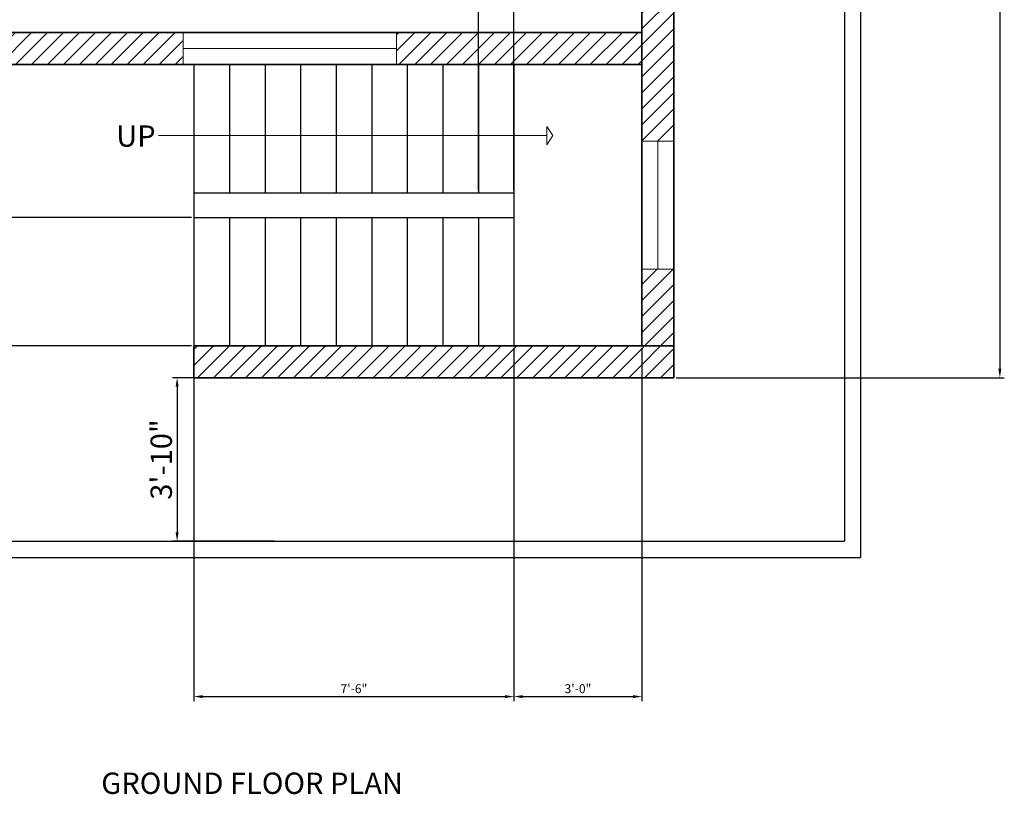
# Model space of a CAD drawing. Units: inches. Extents: x 3618 to 4156, y 1271 to 2023.
# Tile 2 of 5: x 3879 to 4156, y 1271 to 1488. Entities that reach past the tile are written whole.
import ezdxf

# ---------------------------------------------------------------- set-up
doc = ezdxf.new("R2010")
doc.units = ezdxf.units.IN
for name, color, linetype, lineweight in [('A-ANNO-DIMS', 2, 'Continuous', 18), ('A-ANNO-SYMB', 7, 'Continuous', 18), ('A-ANNO-TEXT', 7, 'Continuous', 18), ('A-ANNO-TITL', 7, 'Continuous', 25), ('A-FLOR-STRS', 7, 'Continuous', 25), ('A-GLAZ', 4, 'Continuous', 18), ('A-WALL', 7, 'Continuous', 35), ('A-WALL-PATT', 252, 'Continuous', 13), ('C-PROP', 7, 'Continuous', 25)]:
    doc.layers.add(name, color=color, linetype=linetype, lineweight=lineweight)
doc.styles.get("Standard").update_dxf_attribs({"font": 'arial.ttf'})
doc.dimstyles.new('ISO-25', dxfattribs={"dimtxt": 2.5, "dimasz": 2.5, "dimexe": 1.25, "dimexo": 0.625, "dimtad": 1, "dimdec": 0, "dimlunit": 3, "dimtxsty": 'Standard', "dimcen": 2.5, "dimadec": 0, "dimazin": 0, "dimtfac": 1, "dimtdec": 0, "dimtmove": 0, "dimatfit": 3, "dimfxl": 1, "dimarcsym": 0})

# ---------------------------------------------------------------- blocks, each defined once
blk = doc.blocks.new('*D2')
at = {"layer": 'A-ANNO-DIMS', "color": 0, "lineweight": -2, "transparency": 16777216}
for p, q in [((3942.74, 1387.81), (3922.22, 1387.81)), ((3923.47, 1385.31), (3923.47, 1344.31)), ((3950.79, 1341.81), (3922.22, 1341.81))]:
    blk.add_line(p, q, dxfattribs=at)
at = {"layer": 'A-ANNO-DIMS', "color": 0, "transparency": 16777216}
for points in [[(3923.05, 1385.31), (3923.88, 1385.31), (3923.47, 1387.81)], [(3923.05, 1344.31), (3923.88, 1344.31), (3923.47, 1341.81)]]:
    blk.add_solid(points, dxfattribs=at)
at = {"layer": 'Defpoints', "color": 0, "transparency": 16777216}
for p in [(3943.36, 1387.81), (3923.47, 1341.81), (3951.41, 1341.81)]:
    blk.add_point(p, dxfattribs=at)
at = {"layer": 'A-ANNO-DIMS', "color": 0, "transparency": 16777216, "insert": (3919.78, 1364.81), "char_height": 6, "attachment_point": 5, "rotation": 90}
blk.add_mtext('3\'-10"', dxfattribs=at)
blk = doc.blocks.new('WINDOW-36X9')
for p, q in [((0, 36), (0, 0)), ((9, 36), (0, 36)), ((4.5, 36), (4.5, 0)), ((9, 0), (9, 36)), ((0, 0), (9, 0))]:
    blk.add_line(p, q)
blk = doc.blocks.new('WINDOW-60X9')
for p, q in [((0, 60), (0, 0)), ((9, 60), (0, 60)), ((4.5, 60), (4.5, 0)), ((9, 0), (9, 60)), ((0, 0), (9, 0))]:
    blk.add_line(p, q)
blk = doc.blocks.new('*D50')
at = {"layer": 'A-ANNO-DIMS', "color": 0, "lineweight": -2, "transparency": 16777216}
for p, q in [((3928.19, 1396.19), (3928.19, 1296.91)), ((4018.19, 1396.19), (4018.19, 1296.91)), ((3930.69, 1298.16), (4015.69, 1298.16))]:
    blk.add_line(p, q, dxfattribs=at)
at = {"layer": 'A-ANNO-DIMS', "color": 0, "transparency": 16777216}
for points in [[(3930.69, 1298.58), (3930.69, 1297.74), (3928.19, 1298.16)], [(4015.69, 1298.58), (4015.69, 1297.74), (4018.19, 1298.16)]]:
    blk.add_solid(points, dxfattribs=at)
at = {"layer": 'Defpoints', "color": 0, "transparency": 16777216}
for p in [(3928.19, 1396.81), (4018.19, 1396.81), (4018.19, 1298.16)]:
    blk.add_point(p, dxfattribs=at)
at = {"layer": 'A-ANNO-DIMS', "color": 0, "transparency": 16777216, "insert": (3973.19, 1300.06), "char_height": 2.5, "attachment_point": 5}
blk.add_mtext('7\'-6"', dxfattribs=at)
blk = doc.blocks.new('*D51')
at = {"layer": 'A-ANNO-DIMS', "color": 0, "lineweight": -2, "transparency": 16777216}
for p, q in [((4018.19, 1396.19), (4018.19, 1296.91)), ((4054.19, 1396.19), (4054.19, 1296.91)), ((4020.69, 1298.16), (4051.69, 1298.16))]:
    blk.add_line(p, q, dxfattribs=at)
at = {"layer": 'A-ANNO-DIMS', "color": 0, "transparency": 16777216}
for points in [[(4020.69, 1298.58), (4020.69, 1297.74), (4018.19, 1298.16)], [(4051.69, 1298.58), (4051.69, 1297.74), (4054.19, 1298.16)]]:
    blk.add_solid(points, dxfattribs=at)
at = {"layer": 'Defpoints', "color": 0, "transparency": 16777216}
for p in [(4018.19, 1396.81), (4054.19, 1396.81), (4054.19, 1298.16)]:
    blk.add_point(p, dxfattribs=at)
at = {"layer": 'A-ANNO-DIMS', "color": 0, "transparency": 16777216, "insert": (4036.19, 1300.06), "char_height": 2.5, "attachment_point": 5}
blk.add_mtext('3\'-0"', dxfattribs=at)
blk = doc.blocks.new('*D52')
at = {"layer": 'A-ANNO-DIMS', "color": 0, "lineweight": -2, "transparency": 16777216}
for p, q in [((3927.56, 1432.81), (3622.79, 1432.81)), ((3624.04, 1399.31), (3624.04, 1430.31)), ((3927.56, 1396.81), (3622.79, 1396.81))]:
    blk.add_line(p, q, dxfattribs=at)
at = {"layer": 'A-ANNO-DIMS', "color": 0, "transparency": 16777216}
for points in [[(3623.62, 1430.31), (3624.45, 1430.31), (3624.04, 1432.81)], [(3623.62, 1399.31), (3624.45, 1399.31), (3624.04, 1396.81)]]:
    blk.add_solid(points, dxfattribs=at)
at = {"layer": 'Defpoints', "color": 0, "transparency": 16777216}
for p in [(3624.04, 1432.81), (3928.19, 1432.81), (3928.19, 1396.81)]:
    blk.add_point(p, dxfattribs=at)
at = {"layer": 'A-ANNO-DIMS', "color": 0, "transparency": 16777216, "insert": (3622.14, 1414.81), "char_height": 2.5, "attachment_point": 5, "rotation": 90}
blk.add_mtext('3\'-0"', dxfattribs=at)
blk = doc.blocks.new('*D53')
at = {"layer": 'A-ANNO-DIMS', "color": 0, "lineweight": -2, "transparency": 16777216}
for p, q in [((4008.19, 1440.44), (4008.19, 1974.21)), ((4018.19, 1440.44), (4018.19, 1974.21)), ((4010.69, 1972.96), (4015.69, 1972.96))]:
    blk.add_line(p, q, dxfattribs=at)
at = {"layer": 'A-ANNO-DIMS', "color": 0, "transparency": 16777216}
for points in [[(4010.69, 1973.38), (4010.69, 1972.54), (4008.19, 1972.96)], [(4015.69, 1973.38), (4015.69, 1972.54), (4018.19, 1972.96)]]:
    blk.add_solid(points, dxfattribs=at)
at = {"layer": 'Defpoints', "color": 0, "transparency": 16777216}
for p in [(4018.19, 1972.96), (4008.19, 1439.81), (4018.19, 1439.81)]:
    blk.add_point(p, dxfattribs=at)
at = {"layer": 'A-ANNO-DIMS', "color": 0, "transparency": 16777216, "insert": (4013.19, 1974.86), "char_height": 2.5, "attachment_point": 5}
blk.add_mtext('0\'-10"', dxfattribs=at)
blk = doc.blocks.new('*D56')
at = {"layer": 'A-ANNO-DIMS', "color": 0, "lineweight": -2, "transparency": 16777216}
for p, q in [((4063.81, 1831.81), (4156.09, 1831.81)), ((4154.84, 1829.31), (4154.84, 1390.31)), ((4063.81, 1387.81), (4156.09, 1387.81))]:
    blk.add_line(p, q, dxfattribs=at)
at = {"layer": 'A-ANNO-DIMS', "color": 0, "transparency": 16777216}
for points in [[(4154.42, 1829.31), (4155.25, 1829.31), (4154.84, 1831.81)], [(4154.42, 1390.31), (4155.25, 1390.31), (4154.84, 1387.81)]]:
    blk.add_solid(points, dxfattribs=at)
at = {"layer": 'Defpoints', "color": 0, "transparency": 16777216}
for p in [(4063.19, 1831.81), (4063.19, 1387.81), (4154.84, 1387.81)]:
    blk.add_point(p, dxfattribs=at)
at = {"layer": 'A-ANNO-DIMS', "color": 0, "transparency": 16777216, "insert": (4152.94, 1609.81), "char_height": 2.5, "attachment_point": 5, "rotation": 90}
blk.add_mtext('37\'-0"', dxfattribs=at)

msp = doc.modelspace()

# ---------------------------------------------------------------- hatches: boundary and pattern name
at = {"layer": 'A-WALL-PATT'}
h = msp.add_hatch(dxfattribs=at)
h.set_pattern_fill('ANSI31', color=256)
h.paths.add_polyline_path([(4115.69, 1933.81), (3704.69, 1933.81), (3704.69, 1885.81), (3713.69, 1885.81), (3713.69, 1924.81), (4115.69, 1924.81)])
h.paths.add_polyline_path([(3886.19, 1924.81), (3881.69, 1924.81), (3881.69, 1786.81), (3875.69, 1786.81), (3875.69, 1782.31), (3892.19, 1782.31), (3892.19, 1786.81), (3886.19, 1786.81)])
h.paths.add_polyline_path([(3763.69, 1784.56), (3763.69, 1786.81), (3713.69, 1786.81), (3713.69, 1782.31), (3763.69, 1782.31)], flags=17)
h.paths.add_polyline_path([(3713.69, 1825.81), (3704.69, 1825.81), (3704.69, 1764.31), (3713.69, 1764.31)])
h.paths.add_polyline_path([(3802.19, 1782.31), (3835.69, 1782.31), (3835.69, 1784.56), (3835.69, 1786.81), (3791.69, 1786.81), (3791.69, 1782.31), (3797.69, 1782.31), (3797.69, 1722.31), (3713.69, 1722.31), (3713.69, 1717.81), (3797.69, 1717.81), (3797.69, 1657.81), (3791.69, 1657.81), (3791.69, 1653.31), (3851.69, 1653.31), (3851.69, 1647.31), (3856.19, 1647.31), (3856.19, 1657.81), (3802.19, 1657.81)])
h.paths.add_polyline_path([(3713.69, 1740.31), (3704.69, 1740.31), (3704.69, 1699.81), (3713.69, 1699.81)])
h.paths.add_polyline_path([(3713.69, 1675.81), (3704.69, 1675.81), (3704.69, 1623.31), (3713.69, 1623.31)])
h.paths.add_polyline_path([(3743.18, 1533.31), (3713.69, 1533.31), (3713.69, 1563.31), (3704.69, 1563.31), (3704.69, 1524.31), (3743.18, 1524.31)])
h.paths.add_polyline_path([(3856.19, 1533.31), (3803.18, 1533.31), (3803.18, 1524.31), (3847.19, 1524.31), (3847.19, 1518.31), (3856.19, 1518.31)])
h.paths.add_polyline_path([(3856.19, 1607.31), (3853.94, 1607.31), (3851.69, 1607.31), (3851.69, 1533.31), (3856.19, 1533.31)])
h.paths.add_polyline_path([(3763.69, 1655.56), (3763.69, 1657.81), (3713.69, 1657.81), (3713.69, 1653.31), (3763.69, 1653.31)], flags=17)
h.paths.add_polyline_path([(4063.19, 1670.56), (4054.19, 1670.56), (4054.19, 1645.31), (3940.98, 1645.31), (3940.98, 1640.81), (4054.19, 1640.81), (4054.19, 1592.81), (4063.19, 1592.81)])
h.paths.add_polyline_path([(4063.19, 1532.81), (4054.19, 1532.81), (4054.19, 1454.31), (4063.19, 1454.31)])
h.paths.add_polyline_path([(4054.19, 1484.81), (3985.19, 1484.81), (3985.19, 1475.81), (4054.19, 1475.81)])
h.paths.add_polyline_path([(3925.19, 1484.81), (3856.19, 1484.81), (3856.19, 1490.81), (3847.19, 1490.81), (3847.19, 1475.81), (3925.19, 1475.81)])
h.paths.add_polyline_path([(4063.19, 1396.81), (3928.19, 1396.81), (3928.19, 1387.81), (4063.19, 1387.81)])
h.paths.add_polyline_path([(4063.19, 1418.31), (4054.19, 1418.31), (4054.19, 1396.81), (4063.19, 1396.81)])
h.paths.add_polyline_path([(4063.19, 1790.42), (4054.19, 1790.42), (4054.19, 1786.81), (3932.19, 1786.81), (3932.19, 1784.56), (3932.19, 1782.31), (4054.19, 1782.31), (4054.19, 1771.81), (4063.19, 1771.81)])
h.paths.add_polyline_path([(4070.69, 1840.81), (4058.69, 1840.81), (4058.69, 1890.81), (4056.44, 1890.81), (4054.19, 1890.81), (4054.19, 1826.42), (4063.19, 1826.42), (4063.19, 1831.81), (4070.69, 1831.81)])
h.paths.add_polyline_path([(4115.69, 1924.81), (4106.69, 1924.81), (4106.69, 1840.81), (4094.69, 1840.81), (4094.69, 1831.81), (4115.69, 1831.81)])
h.paths.add_polyline_path([(4063.19, 1731.81), (4058.69, 1731.81), (4054.19, 1731.81), (4054.19, 1706.56), (4063.19, 1706.56)])

# ---------------------------------------------------------------- linework, layer by layer
at = {"layer": 'A-ANNO-SYMB'}
for p, q in [((4027.42, 1455.86), (4027.42, 1458.47)), ((4027.42, 1458.47), (4029.12, 1455.86)), ((3918.28, 1455.86), (4027.42, 1455.86)), ((4027.42, 1455.86), (4027.42, 1453.25)), ((4027.42, 1453.25), (4029.12, 1455.86))]:
    msp.add_line(p, q, dxfattribs=at)
at = {"layer": 'A-FLOR-STRS'}
for p, q in [((3928.19, 1475.81), (3928.19, 1396.81)), ((3938.19, 1475.81), (3938.19, 1439.81)), ((3948.19, 1475.81), (3948.19, 1439.81)), ((3958.19, 1475.81), (3958.19, 1439.81)), ((3968.19, 1475.81), (3968.19, 1439.81)), ((3978.19, 1475.81), (3978.19, 1439.81)), ((3988.19, 1475.81), (3988.19, 1439.81)), ((3998.19, 1475.81), (3998.19, 1439.81)), ((4008.19, 1475.81), (4008.19, 1439.81)), ((4018.19, 1475.81), (4018.19, 1396.81)), ((3928.19, 1439.81), (4018.19, 1439.81)), ((3928.19, 1432.81), (4018.19, 1432.81)), ((3938.19, 1432.81), (3938.19, 1396.81)), ((3948.19, 1432.81), (3948.19, 1396.81)), ((3958.19, 1432.81), (3958.19, 1396.81)), ((3968.19, 1432.81), (3968.19, 1396.81)), ((3978.19, 1432.81), (3978.19, 1396.81)), ((3988.19, 1432.81), (3988.19, 1396.81)), ((3998.19, 1432.81), (3998.19, 1396.81)), ((4008.19, 1432.81), (4008.19, 1396.81))]:
    msp.add_line(p, q, dxfattribs=at)
at = {"layer": 'A-WALL'}
for p, q in [((4063.19, 1831.81), (4063.19, 1387.81)), ((4054.19, 1640.81), (4054.19, 1396.81)), ((3856.19, 1484.81), (4054.19, 1484.81)), ((3847.19, 1475.81), (4054.19, 1475.81)), ((3928.19, 1396.81), (4063.19, 1396.81)), ((3928.19, 1396.81), (3928.19, 1387.81)), ((3928.19, 1387.81), (4063.19, 1387.81))]:
    msp.add_line(p, q, dxfattribs=at)
at = {"layer": 'C-PROP'}
for p, q in [((4115.69, 1933.81), (4115.69, 1341.81)), ((4111.19, 1831.81), (4111.19, 1341.81)), ((3704.69, 1341.81), (4111.19, 1341.81)), ((4115.69, 1341.81), (4115.69, 1337.31)), ((3704.69, 1337.31), (4115.69, 1337.31))]:
    msp.add_line(p, q, dxfattribs=at)

# ---------------------------------------------------------------- block references
at = {"layer": 'A-GLAZ', "rotation": 270.0000000000028}
msp.add_blockref('WINDOW-60X9', (3925.19, 1484.81), dxfattribs=at)
at = {"layer": 'A-GLAZ'}
msp.add_blockref('WINDOW-36X9', (4054.19, 1418.31), dxfattribs=at)

# ---------------------------------------------------------------- texts
at = {"layer": 'A-ANNO-TEXT', "insert": (3906.35, 1458.74), "char_height": 6, "attachment_point": 1}
msp.add_mtext('UP', dxfattribs=at)
at = {"layer": 'A-ANNO-TITL', "insert": (3902.13, 1276.8), "char_height": 6, "attachment_point": 1}
msp.add_mtext('GROUND FLOOR PLAN', dxfattribs=at)

# ---------------------------------------------------------------- dimensions: what is measured, and where the dimension line sits
at = {"layer": 'A-ANNO-DIMS'}
for base, p1, p2, picture, middle in [((4018.19, 1972.96), (4008.19, 1439.81), (4018.19, 1439.81), '*D53', (4013.19, 1974.86)), ((4018.19, 1298.16), (3928.19, 1396.81), (4018.19, 1396.81), '*D50', (3973.19, 1300.06)), ((4054.19, 1298.16), (4018.19, 1396.81), (4054.19, 1396.81), '*D51', (4036.19, 1300.06))]:
    dim = msp.add_linear_dim(base=base, p1=p1, p2=p2, dimstyle='ISO-25', override={"dimdec": 1, "dimlfac": 1, "dimrnd": 0, "dimzin": 1, "dimdsep": 46, "dimlunit": 4, "dimfrac": 2}, dxfattribs=at)
    dim.commit()
    dim.dimension.update_dxf_attribs({"geometry": picture, "text_midpoint": middle})
for base, p1, p2, override, picture, middle in [((4154.84, 1387.81), (4063.19, 1831.81), (4063.19, 1387.81), {"dimdec": 1, "dimlfac": 1, "dimrnd": 0, "dimzin": 1, "dimdsep": 46, "dimlunit": 4, "dimfrac": 2}, '*D56', (4152.94, 1609.81)), ((3624.04, 1432.81), (3928.19, 1396.81), (3928.19, 1432.81), {"dimdec": 1, "dimlfac": 1, "dimrnd": 0, "dimzin": 1, "dimdsep": 46, "dimlunit": 4, "dimfrac": 2}, '*D52', (3622.14, 1414.81)), ((3923.47, 1341.81), (3943.36, 1387.81), (3951.41, 1341.81), {"dimtxt": 6, "dimclrd": 0, "dimclre": 0, "dimclrt": 0}, '*D2', (3919.78, 1364.81))]:
    dim = msp.add_linear_dim(base=base, p1=p1, p2=p2, angle=90, dimstyle='ISO-25', override=override, dxfattribs=at)
    dim.commit()
    dim.dimension.update_dxf_attribs({"geometry": picture, "text_midpoint": middle})

doc.saveas('drawing.dxf')
